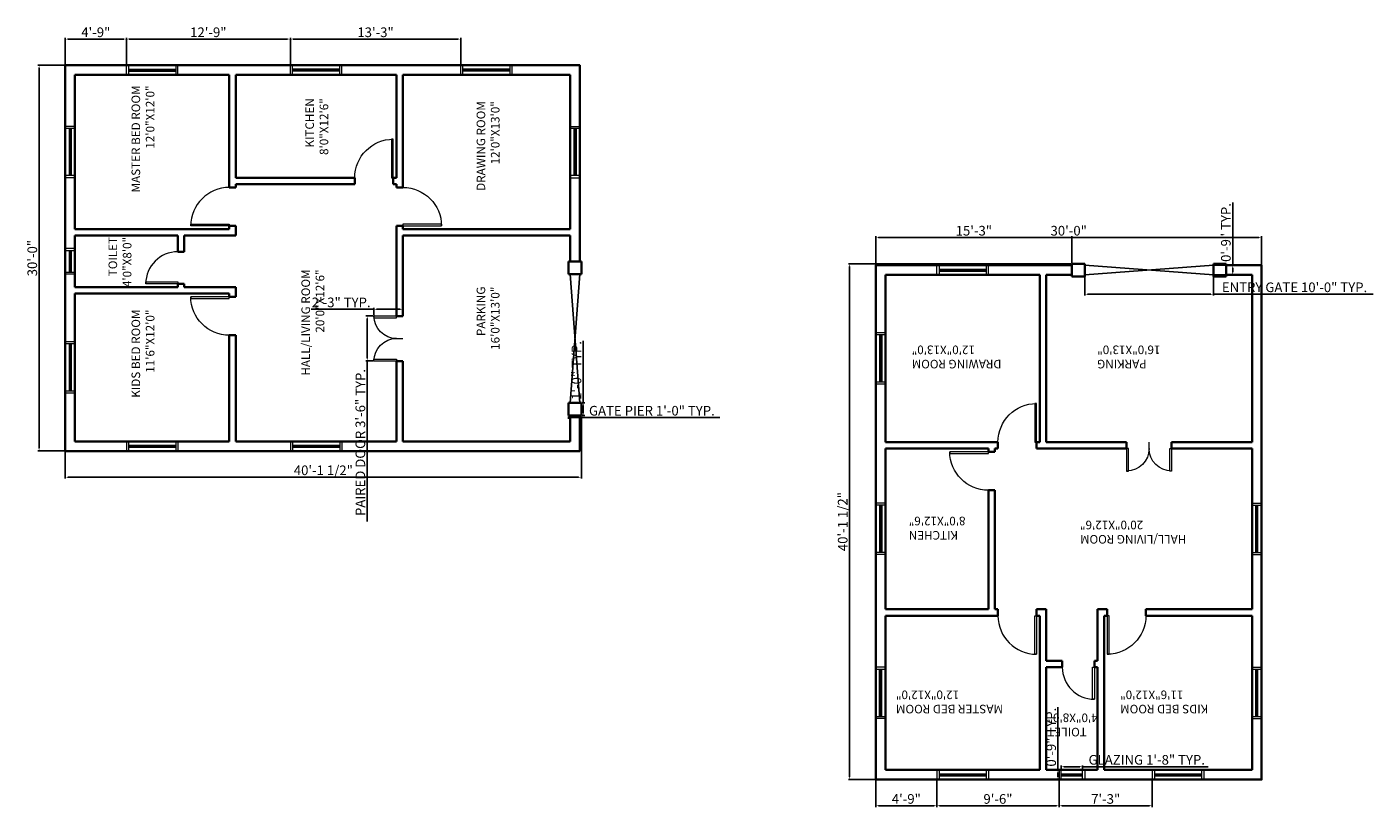
# Model space of a CAD drawing. Units: inches. Extents: x 2639 to 6021, y 292 to 2009.
# Tile 6 of 6: x 4765 to 6021, y 1280 to 2009. Entities that reach past the tile are written whole.
import ezdxf

# ---------------------------------------------------------------- set-up
doc = ezdxf.new("R2010")
doc.units = ezdxf.units.IN
for name, color, linetype, lineweight in [('A-ANNO-DIMS', 2, 'Continuous', 18), ('A-AREA-IDEN', 7, 'Continuous', 18), ('A-COLS', 7, 'Continuous', 35), ('A-DOOR', 3, 'Continuous', 20), ('A-DOOR-GATE', 3, 'Continuous', 25), ('A-GLAZ', 4, 'Continuous', 18), ('A-WALL', 7, 'Continuous', 35)]:
    doc.layers.add(name, color=color, linetype=linetype, lineweight=lineweight)
doc.styles.get("Standard").update_dxf_attribs({"font": 'arial.ttf'})
doc.dimstyles.new('ISO-25', dxfattribs={"dimtxt": 9, "dimasz": 2.5, "dimexe": 1.25, "dimexo": 0.625, "dimtad": 1, "dimdec": 1, "dimlunit": 3, "dimtxsty": 'Standard', "dimcen": 2.5, "dimadec": 0, "dimazin": 0, "dimtfac": 1, "dimtdec": 1, "dimtmove": 0, "dimatfit": 3, "dimfxl": 1, "dimarcsym": 0})

# ---------------------------------------------------------------- blocks, each defined once
blk = doc.blocks.new('*U2')
for p, q in [((0, 0), (0, -6)), ((30, 0), (30, -6))]:
    blk.add_line(p, q)
blk.add_lwpolyline([(0, 0), (0, 30), (1.75, 30), (1.75, 0)], close=True)
blk.add_arc((0, 0), 30, 0, 90)
blk = doc.blocks.new('*U3')
for p, q in [((0, 0), (0, -6)), ((36, 0), (36, -6))]:
    blk.add_line(p, q)
blk.add_lwpolyline([(0, 0), (0, 36), (1.75, 36), (1.75, 0)], close=True)
blk.add_arc((0, 0), 36, 0, 90)
blk = doc.blocks.new('1')
for p, q in [((0, 6), (0, 0)), ((21, 6), (21, 0)), ((21, 6), (21, 0)), ((42, 6), (42, 0))]:
    blk.add_line(p, q)
for points in [[(0, 6), (0, 27), (1.75, 27), (1.75, 6)], [(42, 6), (42, 27), (40.25, 27), (40.25, 6)]]:
    blk.add_lwpolyline(points, close=True)
for centre, start, end in [((0, 6), 0, 90), ((42, 6), 90, 180)]:
    blk.add_arc(centre, 21, start, end)
blk = doc.blocks.new('WINDOW-PLAN-48IN')
for p, q in [((0, 9), (0, 0)), ((0, 5.5), (44, 5.5)), ((0, 4.5), (44, 4.5)), ((0, 3.5), (44, 3.5)), ((44, 9), (44, 0))]:
    blk.add_line(p, q)
blk = doc.blocks.new('WINDOW-PLAN-24IN')
for p, q in [((0, 0), (0, 9)), ((0, 5.5), (20, 5.5)), ((0, 4.5), (20, 4.5)), ((0, 3.5), (20, 3.5)), ((20, 0), (20, 9))]:
    blk.add_line(p, q)
blk = doc.blocks.new('GATE-PIER-12IN')
for p, q in [((0, 12), (12, 12)), ((0, 12), (0, 0)), ((12, 12), (12, 0))]:
    blk.add_line(p, q)
blk.add_lwpolyline([(0, 0), (12, 0)])
blk = doc.blocks.new('GATE-PLAN-10FT')
for p, q in [((0, 9), (120, 0)), ((0, 0), (120, 9))]:
    blk.add_line(p, q)
blk = doc.blocks.new('*D34')
at = {"layer": 'A-ANNO-DIMS', "color": 0, "lineweight": -2, "transparency": 16777216}
for p, q in [((5729.7, 1315.7), (5729.7, 1319.4)), ((5749.7, 1315.7), (5749.7, 1319.4)), ((5732.2, 1318.1), (5747.2, 1318.1)), ((5749.7, 1318.1), (5866.9, 1318.1))]:
    blk.add_line(p, q, dxfattribs=at)
at = {"layer": 'A-ANNO-DIMS', "color": 0, "transparency": 16777216}
for points in [[(5732.2, 1318.5), (5732.2, 1317.7), (5729.7, 1318.1)], [(5747.2, 1318.5), (5747.2, 1317.7), (5749.7, 1318.1)]]:
    blk.add_solid(points, dxfattribs=at)
at = {"layer": 'Defpoints', "color": 0, "transparency": 16777216}
for p in [(5729.7, 1315.1), (5749.7, 1318.1), (5749.7, 1315.1)]:
    blk.add_point(p, dxfattribs=at)
at = {"layer": 'A-ANNO-DIMS', "color": 0, "transparency": 16777216, "insert": (5809.5, 1323.4), "char_height": 9, "attachment_point": 5}
blk.add_mtext('GLAZING 1\'-8" TYP.', dxfattribs=at)
blk = doc.blocks.new('*D35')
at = {"layer": 'A-ANNO-DIMS', "color": 0, "lineweight": -2, "transparency": 16777216}
for p, q in [((5726.7, 1315.1), (5726.7, 1373.7)), ((5729.1, 1315.1), (5725.5, 1315.1)), ((5726.7, 1308.6), (5726.7, 1312.6)), ((5729.1, 1306.1), (5725.5, 1306.1))]:
    blk.add_line(p, q, dxfattribs=at)
at = {"layer": 'A-ANNO-DIMS', "color": 0, "transparency": 16777216}
for points in [[(5726.3, 1312.6), (5727.1, 1312.6), (5726.7, 1315.1)], [(5726.3, 1308.6), (5727.1, 1308.6), (5726.7, 1306.1)]]:
    blk.add_solid(points, dxfattribs=at)
at = {"layer": 'Defpoints', "color": 0, "transparency": 16777216}
for p in [(5726.7, 1315.1), (5729.7, 1315.1), (5729.7, 1306.1)]:
    blk.add_point(p, dxfattribs=at)
at = {"layer": 'A-ANNO-DIMS', "color": 0, "transparency": 16777216, "insert": (5721.5, 1345.7), "char_height": 9, "attachment_point": 5, "rotation": 90}
blk.add_mtext('0\'-9" TYP.', dxfattribs=at)
blk = doc.blocks.new('*D36')
at = {"layer": 'A-ANNO-DIMS', "color": 0, "lineweight": -2, "transparency": 16777216}
for p, q in [((5087.9, 1738.8), (5081, 1738.8)), ((5082.2, 1736.3), (5082.2, 1699.3)), ((5087.9, 1696.8), (5081, 1696.8)), ((5082.2, 1696.8), (5082.2, 1547.1))]:
    blk.add_line(p, q, dxfattribs=at)
at = {"layer": 'A-ANNO-DIMS', "color": 0, "transparency": 16777216}
for points in [[(5081.8, 1736.3), (5082.7, 1736.3), (5082.2, 1738.8)], [(5081.8, 1699.3), (5082.7, 1699.3), (5082.2, 1696.8)]]:
    blk.add_solid(points, dxfattribs=at)
at = {"layer": 'Defpoints', "color": 0, "transparency": 16777216}
for p in [(5088.5, 1738.8), (5082.2, 1696.8), (5088.5, 1696.8)]:
    blk.add_point(p, dxfattribs=at)
at = {"layer": 'A-ANNO-DIMS', "color": 0, "transparency": 16777216, "insert": (5077, 1620.7), "char_height": 9, "attachment_point": 5, "rotation": 90}
blk.add_mtext('PAIRED DOOR 3\'-6" TYP.', dxfattribs=at)
blk = doc.blocks.new('*D37')
at = {"layer": 'A-ANNO-DIMS', "color": 0, "lineweight": -2, "transparency": 16777216}
for p, q in [((5088.5, 1739.4), (5088.5, 1746.3)), ((5115.5, 1739.4), (5115.5, 1746.3)), ((5088.5, 1745.1), (5029.8, 1745.1)), ((5113, 1745.1), (5091, 1745.1))]:
    blk.add_line(p, q, dxfattribs=at)
at = {"layer": 'A-ANNO-DIMS', "color": 0, "transparency": 16777216}
for points in [[(5091, 1745.5), (5091, 1744.6), (5088.5, 1745.1)], [(5113, 1745.5), (5113, 1744.6), (5115.5, 1745.1)]]:
    blk.add_solid(points, dxfattribs=at)
at = {"layer": 'Defpoints', "color": 0, "transparency": 16777216}
for p in [(5088.5, 1745.1), (5088.5, 1738.8), (5115.5, 1738.8)]:
    blk.add_point(p, dxfattribs=at)
at = {"layer": 'A-ANNO-DIMS', "color": 0, "transparency": 16777216, "insert": (5057.9, 1750.3), "char_height": 9, "attachment_point": 5}
blk.add_mtext('2\'-3" TYP.', dxfattribs=at)
blk = doc.blocks.new('*D38')
at = {"layer": 'A-ANNO-DIMS', "color": 0, "lineweight": -2, "transparency": 16777216}
for p, q in [((5751.7, 1776.5), (5751.7, 1757.9)), ((5871.7, 1776.5), (5871.7, 1757.9)), ((5754.2, 1759.1), (5869.2, 1759.1)), ((5871.7, 1759.1), (6020.7, 1759.1))]:
    blk.add_line(p, q, dxfattribs=at)
at = {"layer": 'A-ANNO-DIMS', "color": 0, "transparency": 16777216}
for points in [[(5754.2, 1759.5), (5754.2, 1758.7), (5751.7, 1759.1)], [(5869.2, 1759.5), (5869.2, 1758.7), (5871.7, 1759.1)]]:
    blk.add_solid(points, dxfattribs=at)
at = {"layer": 'Defpoints', "color": 0, "transparency": 16777216}
for p in [(5751.7, 1777.1), (5871.7, 1777.1), (5871.7, 1759.1)]:
    blk.add_point(p, dxfattribs=at)
at = {"layer": 'A-ANNO-DIMS', "color": 0, "transparency": 16777216, "insert": (5947.4, 1764.4), "char_height": 9, "attachment_point": 5}
blk.add_mtext('ENTRY GATE 10\'-0" TYP.', dxfattribs=at)
blk = doc.blocks.new('*D39')
at = {"layer": 'A-ANNO-DIMS', "color": 0, "lineweight": -2, "transparency": 16777216}
for p, q in [((5889.7, 1786.1), (5889.7, 1844.7)), ((5872.3, 1786.1), (5891, 1786.1)), ((5889.7, 1779.6), (5889.7, 1783.6)), ((5872.3, 1777.1), (5891, 1777.1))]:
    blk.add_line(p, q, dxfattribs=at)
at = {"layer": 'A-ANNO-DIMS', "color": 0, "transparency": 16777216}
for points in [[(5889.3, 1783.6), (5890.1, 1783.6), (5889.7, 1786.1)], [(5889.3, 1779.6), (5890.1, 1779.6), (5889.7, 1777.1)]]:
    blk.add_solid(points, dxfattribs=at)
at = {"layer": 'Defpoints', "color": 0, "transparency": 16777216}
for p in [(5871.7, 1786.1), (5889.7, 1786.1), (5871.7, 1777.1)]:
    blk.add_point(p, dxfattribs=at)
at = {"layer": 'A-ANNO-DIMS', "color": 0, "transparency": 16777216, "insert": (5884.5, 1816.7), "char_height": 9, "attachment_point": 5, "rotation": 90}
blk.add_mtext('0\'-9" TYP.', dxfattribs=at)
blk = doc.blocks.new('*D40')
at = {"layer": 'A-ANNO-DIMS', "color": 0, "lineweight": -2, "transparency": 16777216}
for p, q in [((5270, 1645.1), (5270, 1642.7)), ((5272.5, 1644), (5279.5, 1644)), ((5282, 1645.1), (5282, 1642.7)), ((5282, 1644), (5411.1, 1644))]:
    blk.add_line(p, q, dxfattribs=at)
at = {"layer": 'A-ANNO-DIMS', "color": 0, "transparency": 16777216}
for points in [[(5272.5, 1644.4), (5272.5, 1643.5), (5270, 1644)], [(5279.5, 1644.4), (5279.5, 1643.5), (5282, 1644)]]:
    blk.add_solid(points, dxfattribs=at)
at = {"layer": 'Defpoints', "color": 0, "transparency": 16777216}
for p in [(5270, 1645.8), (5282, 1645.8), (5282, 1644)]:
    blk.add_point(p, dxfattribs=at)
at = {"layer": 'A-ANNO-DIMS', "color": 0, "transparency": 16777216, "insert": (5347.8, 1649.2), "char_height": 9, "attachment_point": 5}
blk.add_mtext('GATE PIER 1\'-0" TYP.', dxfattribs=at)
blk = doc.blocks.new('*D41')
at = {"layer": 'A-ANNO-DIMS', "color": 0, "lineweight": -2, "transparency": 16777216}
for p, q in [((5283.8, 1657.8), (5283.8, 1715.5)), ((5282.7, 1657.8), (5285.1, 1657.8)), ((5282.7, 1645.8), (5285.1, 1645.8)), ((5283.8, 1648.3), (5283.8, 1655.3))]:
    blk.add_line(p, q, dxfattribs=at)
at = {"layer": 'A-ANNO-DIMS', "color": 0, "transparency": 16777216}
for points in [[(5283.4, 1655.3), (5284.3, 1655.3), (5283.8, 1657.8)], [(5283.4, 1648.3), (5284.3, 1648.3), (5283.8, 1645.8)]]:
    blk.add_solid(points, dxfattribs=at)
at = {"layer": 'Defpoints', "color": 0, "transparency": 16777216}
for p in [(5282, 1657.8), (5282, 1645.8), (5283.8, 1657.8)]:
    blk.add_point(p, dxfattribs=at)
at = {"layer": 'A-ANNO-DIMS', "color": 0, "transparency": 16777216, "insert": (5278.6, 1687.9), "char_height": 9, "attachment_point": 5, "rotation": 90}
blk.add_mtext('1\'-0" TYP.', dxfattribs=at)
blk = doc.blocks.new('*D50')
at = {"layer": 'A-ANNO-DIMS', "color": 0, "lineweight": -2, "transparency": 16777216}
for p, q in [((5282, 1645.1), (5282, 1587.1)), ((4800.5, 1612.1), (4800.5, 1587.1)), ((4803, 1588.3), (5279.5, 1588.3))]:
    blk.add_line(p, q, dxfattribs=at)
at = {"layer": 'A-ANNO-DIMS', "color": 0, "transparency": 16777216}
for points in [[(4803, 1588.7), (4803, 1587.9), (4800.5, 1588.3)], [(5279.5, 1588.7), (5279.5, 1587.9), (5282, 1588.3)]]:
    blk.add_solid(points, dxfattribs=at)
at = {"layer": 'Defpoints', "color": 0, "transparency": 16777216}
for p in [(5282, 1645.8), (4800.5, 1612.8), (5282, 1588.3)]:
    blk.add_point(p, dxfattribs=at)
at = {"layer": 'A-ANNO-DIMS', "color": 0, "transparency": 16777216, "insert": (5041.3, 1593.6), "char_height": 9, "attachment_point": 5}
blk.add_mtext('40\'-1 1/2"', dxfattribs=at)
blk = doc.blocks.new('*D51')
at = {"layer": 'A-ANNO-DIMS', "color": 0, "lineweight": -2, "transparency": 16777216}
for p, q in [((4799.9, 1972.8), (4774.8, 1972.8)), ((4776.1, 1615.3), (4776.1, 1970.3)), ((4799.9, 1612.8), (4774.8, 1612.8))]:
    blk.add_line(p, q, dxfattribs=at)
at = {"layer": 'A-ANNO-DIMS', "color": 0, "transparency": 16777216}
for points in [[(4775.7, 1970.3), (4776.5, 1970.3), (4776.1, 1972.8)], [(4775.7, 1615.3), (4776.5, 1615.3), (4776.1, 1612.8)]]:
    blk.add_solid(points, dxfattribs=at)
at = {"layer": 'Defpoints', "color": 0, "transparency": 16777216}
for p in [(4776.1, 1972.8), (4800.5, 1972.8), (4800.5, 1612.8)]:
    blk.add_point(p, dxfattribs=at)
at = {"layer": 'A-ANNO-DIMS', "color": 0, "transparency": 16777216, "insert": (4770.9, 1792.8), "char_height": 9, "attachment_point": 5, "rotation": 90}
blk.add_mtext('30\'-0"', dxfattribs=at)
blk = doc.blocks.new('*D52')
at = {"layer": 'A-ANNO-DIMS', "color": 0, "lineweight": -2, "transparency": 16777216}
for p, q in [((5556.7, 1786.7), (5556.7, 1813.3)), ((5559.2, 1812), (5914.2, 1812)), ((5916.7, 1786.7), (5916.7, 1813.3))]:
    blk.add_line(p, q, dxfattribs=at)
at = {"layer": 'A-ANNO-DIMS', "color": 0, "transparency": 16777216}
for points in [[(5559.2, 1812.4), (5559.2, 1811.6), (5556.7, 1812)], [(5914.2, 1812.4), (5914.2, 1811.6), (5916.7, 1812)]]:
    blk.add_solid(points, dxfattribs=at)
at = {"layer": 'Defpoints', "color": 0, "transparency": 16777216}
for p in [(5916.7, 1812), (5556.7, 1786.1), (5916.7, 1786.1)]:
    blk.add_point(p, dxfattribs=at)
at = {"layer": 'A-ANNO-DIMS', "color": 0, "transparency": 16777216, "insert": (5736.7, 1817.2), "char_height": 9, "attachment_point": 5}
blk.add_mtext('30\'-0"', dxfattribs=at)
blk = doc.blocks.new('*D53')
at = {"layer": 'A-ANNO-DIMS', "color": 0, "lineweight": -2, "transparency": 16777216}
for p, q in [((5739.1, 1787.6), (5531.1, 1787.6)), ((5532.3, 1308.6), (5532.3, 1785.1)), ((5556.1, 1306.1), (5531.1, 1306.1))]:
    blk.add_line(p, q, dxfattribs=at)
at = {"layer": 'A-ANNO-DIMS', "color": 0, "transparency": 16777216}
for points in [[(5531.9, 1785.1), (5532.7, 1785.1), (5532.3, 1787.6)], [(5531.9, 1308.6), (5532.7, 1308.6), (5532.3, 1306.1)]]:
    blk.add_solid(points, dxfattribs=at)
at = {"layer": 'Defpoints', "color": 0, "transparency": 16777216}
for p in [(5532.3, 1787.6), (5739.7, 1787.6), (5556.7, 1306.1)]:
    blk.add_point(p, dxfattribs=at)
at = {"layer": 'A-ANNO-DIMS', "color": 0, "transparency": 16777216, "insert": (5527, 1546.9), "char_height": 9, "attachment_point": 5, "rotation": 90}
blk.add_mtext('40\'-1 1/2"', dxfattribs=at)
blk = doc.blocks.new('*D63')
at = {"layer": 'A-ANNO-DIMS', "color": 0, "lineweight": -2, "transparency": 16777216}
for p, q in [((5556.7, 1786.7), (5556.7, 1813.3)), ((5559.2, 1812), (5737.2, 1812)), ((5739.7, 1788.2), (5739.7, 1813.3))]:
    blk.add_line(p, q, dxfattribs=at)
at = {"layer": 'A-ANNO-DIMS', "color": 0, "transparency": 16777216}
for points in [[(5559.2, 1812.4), (5559.2, 1811.6), (5556.7, 1812)], [(5737.2, 1812.4), (5737.2, 1811.6), (5739.7, 1812)]]:
    blk.add_solid(points, dxfattribs=at)
at = {"layer": 'Defpoints', "color": 0, "transparency": 16777216}
for p in [(5739.7, 1812), (5556.7, 1786.1), (5739.7, 1787.6)]:
    blk.add_point(p, dxfattribs=at)
at = {"layer": 'A-ANNO-DIMS', "color": 0, "transparency": 16777216, "insert": (5648.2, 1817.2), "char_height": 9, "attachment_point": 5}
blk.add_mtext('15\'-3"', dxfattribs=at)
blk = doc.blocks.new('*D64')
at = {"layer": 'A-ANNO-DIMS', "color": 0, "lineweight": -2, "transparency": 16777216}
for p, q in [((5556.7, 1305.5), (5556.7, 1280.5)), ((5613.7, 1305.5), (5613.7, 1280.5)), ((5559.2, 1281.7), (5611.2, 1281.7))]:
    blk.add_line(p, q, dxfattribs=at)
at = {"layer": 'A-ANNO-DIMS', "color": 0, "transparency": 16777216}
for points in [[(5559.2, 1282.1), (5559.2, 1281.3), (5556.7, 1281.7)], [(5611.2, 1282.1), (5611.2, 1281.3), (5613.7, 1281.7)]]:
    blk.add_solid(points, dxfattribs=at)
at = {"layer": 'Defpoints', "color": 0, "transparency": 16777216}
for p in [(5556.7, 1306.1), (5613.7, 1306.1), (5613.7, 1281.7)]:
    blk.add_point(p, dxfattribs=at)
at = {"layer": 'A-ANNO-DIMS', "color": 0, "transparency": 16777216, "insert": (5585.2, 1286.9), "char_height": 9, "attachment_point": 5}
blk.add_mtext('4\'-9"', dxfattribs=at)
blk = doc.blocks.new('*D65')
at = {"layer": 'A-ANNO-DIMS', "color": 0, "lineweight": -2, "transparency": 16777216}
for p, q in [((5613.7, 1305.5), (5613.7, 1280.5)), ((5727.7, 1305.5), (5727.7, 1280.5)), ((5616.2, 1281.7), (5725.2, 1281.7))]:
    blk.add_line(p, q, dxfattribs=at)
at = {"layer": 'A-ANNO-DIMS', "color": 0, "transparency": 16777216}
for points in [[(5616.2, 1282.1), (5616.2, 1281.3), (5613.7, 1281.7)], [(5725.2, 1282.1), (5725.2, 1281.3), (5727.7, 1281.7)]]:
    blk.add_solid(points, dxfattribs=at)
at = {"layer": 'Defpoints', "color": 0, "transparency": 16777216}
for p in [(5613.7, 1306.1), (5727.7, 1306.1), (5727.7, 1281.7)]:
    blk.add_point(p, dxfattribs=at)
at = {"layer": 'A-ANNO-DIMS', "color": 0, "transparency": 16777216, "insert": (5670.7, 1286.9), "char_height": 9, "attachment_point": 5}
blk.add_mtext('9\'-6"', dxfattribs=at)
blk = doc.blocks.new('*D66')
at = {"layer": 'A-ANNO-DIMS', "color": 0, "lineweight": -2, "transparency": 16777216}
for p, q in [((5727.7, 1305.5), (5727.7, 1280.5)), ((5814.7, 1305.5), (5814.7, 1280.5)), ((5730.2, 1281.7), (5812.2, 1281.7))]:
    blk.add_line(p, q, dxfattribs=at)
at = {"layer": 'A-ANNO-DIMS', "color": 0, "transparency": 16777216}
for points in [[(5730.2, 1282.1), (5730.2, 1281.3), (5727.7, 1281.7)], [(5812.2, 1282.1), (5812.2, 1281.3), (5814.7, 1281.7)]]:
    blk.add_solid(points, dxfattribs=at)
at = {"layer": 'Defpoints', "color": 0, "transparency": 16777216}
for p in [(5727.7, 1306.1), (5814.7, 1306.1), (5814.7, 1281.7)]:
    blk.add_point(p, dxfattribs=at)
at = {"layer": 'A-ANNO-DIMS', "color": 0, "transparency": 16777216, "insert": (5771.2, 1286.9), "char_height": 9, "attachment_point": 5}
blk.add_mtext('7\'-3"', dxfattribs=at)
blk = doc.blocks.new('*D67')
at = {"layer": 'A-ANNO-DIMS', "color": 0, "lineweight": -2, "transparency": 16777216}
for p, q in [((4800.5, 1973.4), (4800.5, 1998.5)), ((4803, 1997.2), (4855, 1997.2)), ((4857.5, 1973.4), (4857.5, 1998.5))]:
    blk.add_line(p, q, dxfattribs=at)
at = {"layer": 'A-ANNO-DIMS', "color": 0, "transparency": 16777216}
for points in [[(4803, 1997.6), (4803, 1996.8), (4800.5, 1997.2)], [(4855, 1997.6), (4855, 1996.8), (4857.5, 1997.2)]]:
    blk.add_solid(points, dxfattribs=at)
at = {"layer": 'Defpoints', "color": 0, "transparency": 16777216}
for p in [(4857.5, 1997.2), (4800.5, 1972.8), (4857.5, 1972.8)]:
    blk.add_point(p, dxfattribs=at)
at = {"layer": 'A-ANNO-DIMS', "color": 0, "transparency": 16777216, "insert": (4829, 2002.4), "char_height": 9, "attachment_point": 5}
blk.add_mtext('4\'-9"', dxfattribs=at)
blk = doc.blocks.new('*D68')
at = {"layer": 'A-ANNO-DIMS', "color": 0, "lineweight": -2, "transparency": 16777216}
for p, q in [((4857.5, 1973.4), (4857.5, 1998.5)), ((4860, 1997.2), (5008, 1997.2)), ((5010.5, 1973.4), (5010.5, 1998.5))]:
    blk.add_line(p, q, dxfattribs=at)
at = {"layer": 'A-ANNO-DIMS', "color": 0, "transparency": 16777216}
for points in [[(4860, 1997.6), (4860, 1996.8), (4857.5, 1997.2)], [(5008, 1997.6), (5008, 1996.8), (5010.5, 1997.2)]]:
    blk.add_solid(points, dxfattribs=at)
at = {"layer": 'Defpoints', "color": 0, "transparency": 16777216}
for p in [(5010.5, 1997.2), (4857.5, 1972.8), (5010.5, 1972.8)]:
    blk.add_point(p, dxfattribs=at)
at = {"layer": 'A-ANNO-DIMS', "color": 0, "transparency": 16777216, "insert": (4934, 2002.4), "char_height": 9, "attachment_point": 5}
blk.add_mtext('12\'-9"', dxfattribs=at)
blk = doc.blocks.new('*D69')
at = {"layer": 'A-ANNO-DIMS', "color": 0, "lineweight": -2, "transparency": 16777216}
for p, q in [((5010.5, 1973.4), (5010.5, 1998.5)), ((5013, 1997.2), (5167, 1997.2)), ((5169.5, 1973.4), (5169.5, 1998.5))]:
    blk.add_line(p, q, dxfattribs=at)
at = {"layer": 'A-ANNO-DIMS', "color": 0, "transparency": 16777216}
for points in [[(5013, 1997.6), (5013, 1996.8), (5010.5, 1997.2)], [(5167, 1997.6), (5167, 1996.8), (5169.5, 1997.2)]]:
    blk.add_solid(points, dxfattribs=at)
at = {"layer": 'Defpoints', "color": 0, "transparency": 16777216}
for p in [(5169.5, 1997.2), (5010.5, 1972.8), (5169.5, 1972.8)]:
    blk.add_point(p, dxfattribs=at)
at = {"layer": 'A-ANNO-DIMS', "color": 0, "transparency": 16777216, "insert": (5090, 2002.4), "char_height": 9, "attachment_point": 5}
blk.add_mtext('13\'-3"', dxfattribs=at)

msp = doc.modelspace()

# ---------------------------------------------------------------- linework, layer by layer
at = {"layer": 'A-GLAZ'}
for p, q in [((4857.55, 1963.77), (4857.55, 1972.77)), ((4905.55, 1963.77), (4905.55, 1972.77)), ((5010.55, 1963.77), (5010.55, 1972.77)), ((5058.55, 1963.77), (5058.55, 1972.77)), ((5169.55, 1963.77), (5169.55, 1972.77)), ((5217.55, 1963.77), (5217.55, 1972.77)), ((4809.55, 1915.77), (4800.55, 1915.77)), ((5271.55, 1915.77), (5280.55, 1915.77)), ((4809.55, 1867.77), (4800.55, 1867.77)), ((5271.55, 1867.77), (5280.55, 1867.77)), ((4809.55, 1801.77), (4800.55, 1801.77)), ((5613.71, 1777.1), (5613.71, 1786.1)), ((5661.71, 1777.1), (5661.71, 1786.1)), ((4809.55, 1777.77), (4800.55, 1777.77)), ((5565.71, 1723.1), (5556.71, 1723.1)), ((4809.55, 1714.77), (4800.55, 1714.77)), ((5565.71, 1675.1), (5556.71, 1675.1)), ((4809.55, 1666.77), (4800.55, 1666.77)), ((4857.55, 1621.77), (4857.55, 1612.77)), ((4905.55, 1621.77), (4905.55, 1612.77)), ((5010.55, 1621.77), (5010.55, 1612.77)), ((5058.55, 1621.77), (5058.55, 1612.77)), ((5565.71, 1564.1), (5556.71, 1564.1)), ((5907.71, 1564.1), (5916.71, 1564.1)), ((5565.71, 1516.1), (5556.71, 1516.1)), ((5907.71, 1516.1), (5916.71, 1516.1)), ((5565.71, 1411.1), (5556.71, 1411.1)), ((5907.71, 1411.1), (5916.71, 1411.1)), ((5565.71, 1363.1), (5556.71, 1363.1)), ((5907.71, 1363.1), (5916.71, 1363.1)), ((5613.71, 1315.1), (5613.71, 1306.1)), ((5661.71, 1315.1), (5661.71, 1306.1)), ((5727.71, 1315.1), (5727.71, 1306.1)), ((5751.71, 1315.1), (5751.71, 1306.1)), ((5814.71, 1315.1), (5814.71, 1306.1)), ((5862.71, 1315.1), (5862.71, 1306.1))]:
    msp.add_line(p, q, dxfattribs=at)
at = {"layer": 'A-WALL'}
for p, q in [((4809.55, 1819.77), (4809.55, 1963.77)), ((4809.55, 1963.77), (4953.55, 1963.77)), ((4953.55, 1858.77), (4953.55, 1963.77)), ((4959.55, 1867.77), (4959.55, 1963.77)), ((4959.55, 1963.77), (5109.55, 1963.77)), ((5109.55, 1867.77), (5109.55, 1963.77)), ((5115.55, 1858.77), (5115.55, 1963.77)), ((5115.55, 1963.77), (5271.55, 1963.77)), ((5271.55, 1963.77), (5271.55, 1819.77)), ((4959.55, 1867.77), (5070.55, 1867.77)), ((4959.55, 1858.77), (4959.55, 1861.77)), ((4959.55, 1861.77), (5070.55, 1861.77)), ((5070.55, 1861.77), (5070.55, 1867.77)), ((5106.55, 1861.77), (5106.55, 1867.77)), ((5106.55, 1867.77), (5109.55, 1867.77)), ((5106.55, 1861.77), (5109.55, 1861.77)), ((5109.55, 1858.77), (5109.55, 1861.77)), ((4953.55, 1858.77), (4959.55, 1858.77)), ((5109.55, 1858.77), (5115.55, 1858.77)), ((4953.55, 1819.77), (4953.55, 1822.77)), ((4953.55, 1822.77), (4959.55, 1822.77)), ((4959.55, 1813.77), (4959.55, 1822.77)), ((5109.55, 1738.77), (5109.55, 1822.77)), ((5109.55, 1822.77), (5115.55, 1822.77)), ((5115.55, 1819.77), (5115.55, 1822.77)), ((4809.55, 1819.77), (4953.55, 1819.77)), ((4809.55, 1765.77), (4809.55, 1813.77)), ((4809.55, 1813.77), (4905.55, 1813.77)), ((4905.55, 1798.77), (4905.55, 1813.77)), ((4911.55, 1798.77), (4911.55, 1813.77)), ((4911.55, 1813.77), (4959.55, 1813.77)), ((5115.55, 1819.77), (5271.55, 1819.77)), ((5115.55, 1738.77), (5115.55, 1813.77)), ((5115.55, 1813.77), (5271.55, 1813.77)), ((5271.55, 1813.77), (5271.55, 1789.77)), ((4905.55, 1798.77), (4911.55, 1798.77)), ((5565.71, 1777.1), (5709.71, 1777.1)), ((5565.71, 1621.1), (5565.71, 1777.1)), ((5709.71, 1621.1), (5709.71, 1777.1)), ((5715.71, 1777.1), (5739.71, 1777.1)), ((5715.71, 1621.1), (5715.71, 1777.1)), ((5883.71, 1777.1), (5907.71, 1777.1)), ((5907.71, 1777.1), (5907.71, 1621.1)), ((4809.55, 1765.77), (4905.55, 1765.77)), ((4809.55, 1621.77), (4809.55, 1759.77)), ((4809.55, 1759.77), (4953.55, 1759.77)), ((4905.55, 1765.77), (4905.55, 1768.77)), ((4905.55, 1768.77), (4911.55, 1768.77)), ((4911.55, 1765.77), (4911.55, 1768.77)), ((4911.55, 1765.77), (4959.55, 1765.77)), ((4953.55, 1756.77), (4953.55, 1759.77)), ((4959.55, 1756.77), (4959.55, 1765.77)), ((4953.55, 1756.77), (4959.55, 1756.77)), ((5115.55, 1738.77), (5109.55, 1738.77)), ((4953.55, 1621.77), (4953.55, 1720.77)), ((4953.55, 1720.77), (4959.55, 1720.77)), ((4959.55, 1621.77), (4959.55, 1720.77)), ((5109.55, 1621.77), (5109.55, 1696.77)), ((5115.55, 1696.77), (5109.55, 1696.77)), ((5115.55, 1621.77), (5115.55, 1696.77)), ((5271.55, 1645.77), (5271.55, 1621.77)), ((4953.55, 1621.77), (4809.55, 1621.77)), ((5109.55, 1621.77), (4959.55, 1621.77)), ((5271.55, 1621.77), (5115.55, 1621.77)), ((5670.71, 1621.1), (5565.71, 1621.1)), ((5670.71, 1615.1), (5670.71, 1621.1)), ((5709.71, 1621.1), (5706.71, 1621.1)), ((5706.71, 1615.1), (5706.71, 1621.1)), ((5790.71, 1621.1), (5715.71, 1621.1)), ((5790.71, 1621.1), (5790.71, 1615.1)), ((5907.71, 1621.1), (5832.71, 1621.1)), ((5832.71, 1621.1), (5832.71, 1615.1)), ((5661.71, 1615.1), (5565.71, 1615.1)), ((5565.71, 1465.1), (5565.71, 1615.1)), ((5661.71, 1612.1), (5661.71, 1615.1)), ((5667.71, 1612.1), (5661.71, 1612.1)), ((5670.71, 1615.1), (5667.71, 1615.1)), ((5667.71, 1612.1), (5667.71, 1615.1)), ((5790.71, 1615.1), (5706.71, 1615.1)), ((5907.71, 1615.1), (5832.71, 1615.1)), ((5907.71, 1615.1), (5907.71, 1465.1)), ((5667.71, 1576.1), (5661.71, 1576.1)), ((5661.71, 1465.1), (5661.71, 1576.1)), ((5667.71, 1465.1), (5667.71, 1576.1)), ((5661.71, 1465.1), (5565.71, 1465.1)), ((5670.71, 1459.1), (5565.71, 1459.1)), ((5565.71, 1315.1), (5565.71, 1459.1)), ((5670.71, 1465.1), (5667.71, 1465.1)), ((5670.71, 1459.1), (5670.71, 1465.1)), ((5715.71, 1465.1), (5706.71, 1465.1)), ((5706.71, 1459.1), (5706.71, 1465.1)), ((5709.71, 1459.1), (5706.71, 1459.1)), ((5709.71, 1315.1), (5709.71, 1459.1)), ((5715.71, 1417.1), (5715.71, 1465.1)), ((5772.71, 1465.1), (5763.71, 1465.1)), ((5763.71, 1417.1), (5763.71, 1465.1)), ((5772.71, 1459.1), (5769.71, 1459.1)), ((5769.71, 1315.1), (5769.71, 1459.1)), ((5772.71, 1459.1), (5772.71, 1465.1)), ((5907.71, 1465.1), (5808.71, 1465.1)), ((5808.71, 1459.1), (5808.71, 1465.1)), ((5907.71, 1459.1), (5808.71, 1459.1)), ((5907.71, 1459.1), (5907.71, 1315.1)), ((5730.71, 1417.1), (5715.71, 1417.1)), ((5730.71, 1411.1), (5715.71, 1411.1)), ((5715.71, 1315.1), (5715.71, 1411.1)), ((5730.71, 1411.1), (5730.71, 1417.1)), ((5763.71, 1417.1), (5760.71, 1417.1)), ((5760.71, 1411.1), (5760.71, 1417.1)), ((5763.71, 1411.1), (5760.71, 1411.1)), ((5763.71, 1315.1), (5763.71, 1411.1)), ((5709.71, 1315.1), (5565.71, 1315.1)), ((5763.71, 1315.1), (5715.71, 1315.1)), ((5907.71, 1315.1), (5769.71, 1315.1))]:
    msp.add_line(p, q, dxfattribs=at)
for points in [[(5280.55, 1645.77), (5280.55, 1612.77), (4800.55, 1612.77), (4800.55, 1972.77), (5280.55, 1972.77), (5280.55, 1789.77)], [(5883.71, 1786.1), (5916.71, 1786.1), (5916.71, 1306.1), (5556.71, 1306.1), (5556.71, 1786.1), (5739.71, 1786.1)]]:
    msp.add_lwpolyline(points, dxfattribs=at)

# ---------------------------------------------------------------- block references
at = {"layer": 'A-COLS'}
for p in [(5270.05, 1777.76), (5270.05, 1645.76)]:
    msp.add_blockref('GATE-PIER-12IN', p, dxfattribs=at)
for p, rotation in [((5751.71, 1775.6), 90.00000000000435), ((5883.71, 1775.6), 90.00000000000325)]:
    msp.add_blockref('GATE-PIER-12IN', p, dxfattribs=dict(at, rotation=rotation))
at = {"layer": 'A-DOOR', "xscale": -1}
for p in [(5106.56, 1867.77), (5706.71, 1621.1)]:
    msp.add_blockref('*U3', p, dxfattribs=at)
at = {"layer": 'A-DOOR'}
for name, p, rotation in [('*U3', (4953.55, 1822.77), 90.00000000000003), ('*U2', (4905.55, 1768.77), 90.00000000000003), ('*U3', (5706.71, 1459.1), 180), ('*U2', (5760.71, 1411.1), 180)]:
    msp.add_blockref(name, p, dxfattribs=dict(at, rotation=rotation))
at = {"layer": 'A-DOOR', "xscale": -1}
for name, p, rotation in [('*U3', (5115.55, 1822.77), 270), ('*U3', (4953.55, 1756.77), 90), ('1', (5115.55, 1738.77), 90), ('1', (5790.71, 1621.1), 180), ('*U3', (5661.71, 1612.12), 90), ('*U3', (5772.71, 1459.1), 180)]:
    msp.add_blockref(name, p, dxfattribs=dict(at, rotation=rotation))
at = {"layer": 'A-DOOR-GATE'}
msp.add_blockref('GATE-PLAN-10FT', (5751.71, 1777.1), dxfattribs=at)
at = {"layer": 'A-DOOR-GATE', "rotation": 270}
msp.add_blockref('GATE-PLAN-10FT', (5271.55, 1777.77), dxfattribs=at)
at = {"layer": 'A-GLAZ'}
for name, p in [('WINDOW-PLAN-48IN', (4859.55, 1963.76)), ('WINDOW-PLAN-48IN', (5615.71, 1777.1)), ('WINDOW-PLAN-48IN', (4859.55, 1612.76)), ('WINDOW-PLAN-48IN', (5012.55, 1612.76)), ('WINDOW-PLAN-48IN', (5615.71, 1306.1)), ('WINDOW-PLAN-24IN', (5729.71, 1306.1)), ('WINDOW-PLAN-48IN', (5816.71, 1306.1))]:
    msp.add_blockref(name, p, dxfattribs=at)
for name, p, rotation in [('WINDOW-PLAN-48IN', (5056.55, 1972.77), 180), ('WINDOW-PLAN-48IN', (5215.55, 1972.77), 180), ('WINDOW-PLAN-48IN', (4800.55, 1913.77), 269.999999999995), ('WINDOW-PLAN-48IN', (5271.55, 1913.77), 269.9999999999973), ('WINDOW-PLAN-24IN', (4800.55, 1799.77), 269.9999999999973), ('WINDOW-PLAN-48IN', (5556.71, 1721.1), 269.9999999999974), ('WINDOW-PLAN-48IN', (4800.55, 1712.77), 269.9999999999949), ('WINDOW-PLAN-48IN', (5556.71, 1562.1), 269.9999999999974), ('WINDOW-PLAN-48IN', (5916.71, 1518.1), 89.99999999999979), ('WINDOW-PLAN-48IN', (5565.71, 1365.1), 90.00000000000193), ('WINDOW-PLAN-48IN', (5916.71, 1365.1), 89.99999999999979)]:
    msp.add_blockref(name, p, dxfattribs=dict(at, rotation=rotation))

# ---------------------------------------------------------------- texts
at = {"layer": 'A-AREA-IDEN', "char_height": 8, "attachment_point": 3}
for s, insert, rotation in [('{\\fTimes New Roman|b0|i0|c0|p18;MASTER BED ROOM\\P          12\'0"X12\'0"}', (4862.35, 1953.96), 90), ('{\\fTimes New Roman|b0|i0|c0|p18;KITCHEN\\P8\'0"X12\'6"}', (5024.53, 1942.01), 90), ('{\\fTimes New Roman|b0|i0|c0|p18;DRAWING ROOM\\P      12\'0"X13\'0"}', (5184.31, 1939.26), 90), ('{\\fTimes New Roman|b0|i0|c0|p18;TOILET\\P4\'0"X8\'0"}', (4840.88, 1812.61), 90), ('{\\fTimes New Roman|b0|i0|c0|p18;HALL/LIVING ROOM\\P        20\'0"X12\'6"}', (5020.84, 1782.24), 90), ('{\\fTimes New Roman|b0|i0|c0|p18;PARKING\\P16\'0"X13\'0"}', (5184.31, 1766.18), 90), ('{\\fTimes New Roman|b0|i0|c0|p18;KIDS BED ROOM\\P       11\'6"X12\'0"}', (4862.35, 1744.78), 90), ('{\\fTimes New Roman|b0|i0|c0|p18;DRAWING ROOM\\P      12\'0"X13\'0"}', (5590.21, 1689.87), 180), ('{\\fTimes New Roman|b0|i0|c0|p18;PARKING\\P16\'0"X13\'0"}', (5763.29, 1689.87), 180), ('{\\fTimes New Roman|b0|i0|c0|p18;KITCHEN\\P8\'0"X12\'6"}', (5587.46, 1530.09), 180), ('{\\fTimes New Roman|b0|i0|c0|p18;HALL/LIVING ROOM\\P        20\'0"X12\'6"}', (5747.23, 1526.39), 180), ('{\\fTimes New Roman|b0|i0|c0|p18;MASTER BED ROOM\\P          12\'0"X12\'0"}', (5575.51, 1367.91), 180), ('{\\fTimes New Roman|b0|i0|c0|p18;KIDS BED ROOM\\P       11\'6"X12\'0"}', (5784.69, 1367.91), 180), ('{\\fTimes New Roman|b0|i0|c0|p18;TOILET\\P4\'0"X8\'0"}', (5716.86, 1346.44), 180)]:
    msp.add_mtext_dynamic_manual_height_columns(s, width=172.2916, gutter_width=12.5, heights=[0], dxfattribs=dict(at, insert=insert, rotation=rotation))

# ---------------------------------------------------------------- dimensions: what is measured, and where the dimension line sits
at = {"layer": 'A-ANNO-DIMS'}
for base, p1, p2, picture, middle in [((4857.55, 1997.22), (4800.55, 1972.77), (4857.55, 1972.77), '*D67', (4829.05, 2002.44)), ((5010.55, 1997.22), (4857.55, 1972.77), (5010.55, 1972.77), '*D68', (4934.05, 2002.44)), ((5169.55, 1997.22), (5010.55, 1972.77), (5169.55, 1972.77), '*D69', (5090.05, 2002.44)), ((5916.71, 1812), (5556.71, 1786.1), (5916.71, 1786.1), '*D52', (5736.71, 1817.23)), ((5739.71, 1812), (5556.71, 1786.1), (5739.71, 1787.6), '*D63', (5648.21, 1817.23)), ((5282.05, 1588.32), (4800.55, 1612.77), (5282.05, 1645.77), '*D50', (5041.3, 1593.59)), ((5613.71, 1281.7), (5556.71, 1306.1), (5613.71, 1306.1), '*D64', (5585.21, 1286.92)), ((5727.71, 1281.7), (5613.71, 1306.1), (5727.71, 1306.1), '*D65', (5670.71, 1286.92)), ((5814.71, 1281.7), (5727.71, 1306.1), (5814.71, 1306.1), '*D66', (5771.21, 1286.93))]:
    dim = msp.add_linear_dim(base=base, p1=p1, p2=p2, dimstyle='ISO-25', override={"dimdec": 1, "dimlfac": 1, "dimrnd": 0, "dimzin": 1, "dimdsep": 46, "dimlunit": 4, "dimfrac": 2}, dxfattribs=at)
    dim.commit()
    dim.dimension.update_dxf_attribs({"geometry": picture, "text_midpoint": middle})
for base, p1, p2, picture, middle in [((4776.1, 1972.77), (4800.55, 1612.77), (4800.55, 1972.77), '*D51', (4770.87, 1792.77)), ((5532.31, 1787.6), (5556.71, 1306.1), (5739.71, 1787.6), '*D53', (5527.03, 1546.85))]:
    dim = msp.add_linear_dim(base=base, p1=p1, p2=p2, angle=90, dimstyle='ISO-25', override={"dimdec": 1, "dimlfac": 1, "dimrnd": 0, "dimzin": 1, "dimdsep": 46, "dimlunit": 4, "dimfrac": 2}, dxfattribs=at)
    dim.commit()
    dim.dimension.update_dxf_attribs({"geometry": picture, "text_midpoint": middle})
for base, p1, p2, angle, text, picture, middle in [((5889.71, 1786.1), (5871.71, 1777.1), (5871.71, 1786.1), 90, '<> TYP.', '*D39', (5884.49, 1816.66)), ((5088.55, 1745.07), (5115.55, 1738.77), (5088.55, 1738.77), 180, '<> TYP.', '*D37', (5057.92, 1750.29)), ((5082.25, 1696.77), (5088.55, 1738.77), (5088.55, 1696.77), 270, 'PAIRED DOOR <> TYP.', '*D36', (5076.96, 1620.68)), ((5283.85, 1657.77), (5282.05, 1645.77), (5282.05, 1657.77), 90, '<> TYP.', '*D41', (5278.63, 1687.9)), ((5726.71, 1315.1), (5729.71, 1306.1), (5729.71, 1315.1), 90, '<> TYP.', '*D35', (5721.49, 1345.66))]:
    dim = msp.add_linear_dim(base=base, p1=p1, p2=p2, angle=angle, text=text, dimstyle='ISO-25', override={"dimdec": 1, "dimlfac": 1, "dimrnd": 0, "dimzin": 1, "dimdsep": 46, "dimlunit": 4, "dimfrac": 2}, dxfattribs=at)
    dim.commit()
    dim.dimension.update_dxf_attribs({"geometry": picture, "text_midpoint": middle})
for base, p1, p2, text, picture, middle in [((5871.71, 1759.1), (5751.71, 1777.1), (5871.71, 1777.1), 'ENTRY GATE <> TYP.', '*D38', (5947.44, 1764.38)), ((5282.05, 1643.97), (5270.05, 1645.77), (5282.05, 1645.77), 'GATE PIER <> TYP.', '*D40', (5347.81, 1649.24)), ((5749.71, 1318.1), (5729.71, 1315.1), (5749.71, 1315.1), 'GLAZING <> TYP.', '*D34', (5809.53, 1323.38))]:
    dim = msp.add_linear_dim(base=base, p1=p1, p2=p2, text=text, dimstyle='ISO-25', override={"dimdec": 1, "dimlfac": 1, "dimrnd": 0, "dimzin": 1, "dimdsep": 46, "dimlunit": 4, "dimfrac": 2}, dxfattribs=at)
    dim.commit()
    dim.dimension.update_dxf_attribs({"geometry": picture, "text_midpoint": middle})

doc.saveas('drawing.dxf')
